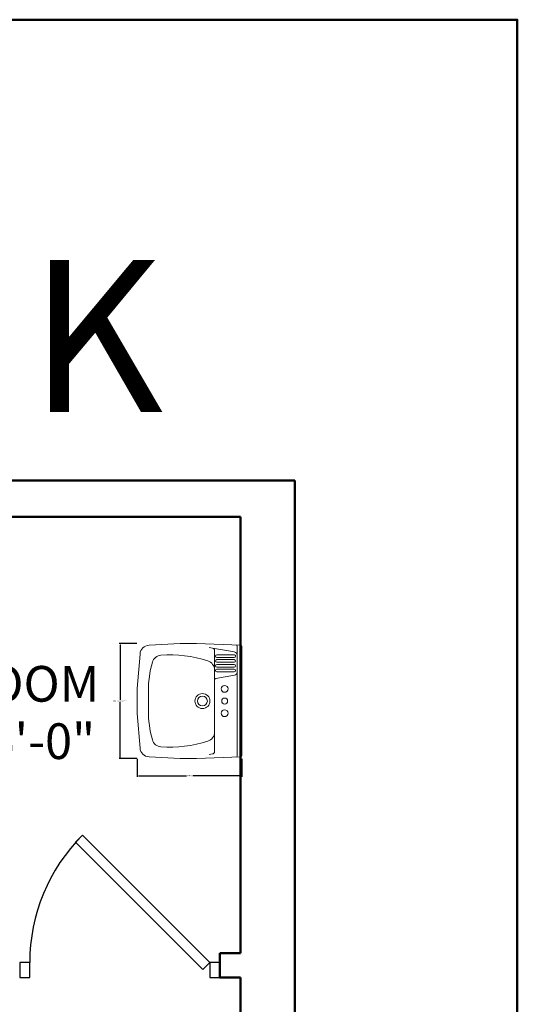
# Model space of a CAD drawing. Units: inches. Extents: x 64 to 1167, y 117 to 939.
# Tile 27 of 56: x 431 to 513, y 777 to 939. Entities that reach past the tile are written whole.
import ezdxf

# ---------------------------------------------------------------- set-up
doc = ezdxf.new("R2010")
doc.units = ezdxf.units.IN
doc.header["$MEASUREMENT"] = 0
for name, color, linetype, lineweight in [('A-ANNO-DIMS', 2, 'Continuous', 18), ('A-ANNO-TEXT', 7, 'Continuous', 25), ('A-ANNO-TTLB', 7, 'Continuous', 50), ('A-DOOR', 4, 'Continuous', 25), ('A-FLOR-FIXT', 8, 'Continuous', 18), ('A-WALL', 7, 'Continuous', 50)]:
    doc.layers.add(name, color=color, linetype=linetype, lineweight=lineweight)
doc.styles.get("Standard").update_dxf_attribs({"font": 'arial.ttf'})
doc.dimstyles.get("Standard").update_dxf_attribs({"dimtxt": 0.18, "dimasz": 0.18, "dimexe": 0.18, "dimexo": 0.0625, "dimgap": 0.09, "dimtad": 0, "dimtih": 1, "dimtoh": 1, "dimdec": 4, "dimzin": 0, "dimdsep": 46, "dimtxsty": 'Standard', "dimcen": 0.09, "dimadec": 0, "dimazin": 0, "dimtfac": 1, "dimtdec": 4, "dimtofl": 0, "dimtmove": 0, "dimatfit": 3, "dimfxl": 1, "dimtolj": 1, "dimtzin": 0, "dimarcsym": 0})

# ---------------------------------------------------------------- blocks, each defined once
blk = doc.blocks.new('A$C68901CC0')
for p, q in [((10.95, 26.62), (12.35, 28.01)), ((12.35, 28.01), (37.4, 2.95)), ((36.01, 1.56), (10.95, 26.62)), ((0, 2.95), (0, 0)), ((1.97, 2.95), (0, 2.95)), ((1.97, 0), (1.97, 2.95)), ((37.4, 2.95), (36.01, 1.56)), ((37.4, 2.95), (37.4, 0)), ((39.37, 2.95), (37.4, 2.95)), ((39.37, 0), (39.37, 2.95)), ((0, 0), (1.97, 0)), ((37.4, 0), (39.37, 0))]:
    blk.add_line(p, q)
blk.add_arc((37.4, 2.95), 35.43, 135, 180)
blk = doc.blocks.new('A$C056A4ABE')
at = {"ltscale": 20}
for p, q in [((0.0065, 0.4339), (0, 0.2479)), ((0.0098, 0.4178), (0.2406, 0.4178)), ((0.2406, 0.4378), (0.0105, 0.4378)), ((0.1205, 0.4178), (0.0475, 0.4178)), ((0.11, 0.4178), (0.0579, 0.4178)), ((0.2406, 0.4378), (0.4708, 0.4378)), ((0.4715, 0.4178), (0.2406, 0.4178)), ((0.4748, 0.4339), (0.4813, 0.2479)), ((0.0188, 0.315), (0.0351, 0.4075)), ((0.0472, 0.4063), (0.0472, 0.3333)), ((0.0582, 0.4063), (0.0582, 0.3333)), ((0.0672, 0.4063), (0.0672, 0.3333)), ((0.0782, 0.4063), (0.0782, 0.3333)), ((0.0872, 0.4063), (0.0872, 0.3333)), ((0.0982, 0.4063), (0.0982, 0.3333)), ((0.1072, 0.4063), (0.1072, 0.3333)), ((0.1182, 0.4063), (0.1182, 0.3333)), ((0.1465, 0.3295), (0.1328, 0.4075)), ((0.0164, 0.3013), (0.0188, 0.315)), ((0.2406, 0.3233), (0.0287, 0.3233)), ((0.2406, 0.3233), (0.1468, 0.3233)), ((0.2406, 0.3233), (0.3344, 0.3233)), ((0.2406, 0.3233), (0.4526, 0.3233)), ((0.4648, 0.3013), (0.4624, 0.315)), ((0, 0.2479), (0, 0.1789)), ((0.4813, 0.2479), (0.4813, 0.1789)), ((0, 0.1789), (0.0068, 0.0492)), ((0.4813, 0.1789), (0.4745, 0.0492)), ((0.2406, 0.0463), (0.2011, 0.0463)), ((0.2406, 0.0463), (0.2802, 0.0463)), ((0.0436, 0.0114), (0.1881, 0)), ((0.1881, 0), (0.2406, 0)), ((0.2932, 0), (0.2406, 0)), ((0.4377, 0.0114), (0.2932, 0))]:
    blk.add_line(p, q, dxfattribs=at)
for centre, radius in [((0.1896, 0.3658), 0.0143), ((0.2406, 0.3658), 0.0125), ((0.2916, 0.3658), 0.0143), ((0.2406, 0.2728), 0.0315), ((0.2406, 0.2728), 0.0205)]:
    blk.add_circle(centre, radius, dxfattribs=at)
for centre, radius, start, end in [((0.0098, 0.4138), 0.004, 90, 178), ((0.0105, 0.4338), 0.004, 90, 178), ((0.0475, 0.4053), 0.0125, 90, 170), ((0.1205, 0.4053), 0.0125, 10, 90), ((0.4708, 0.4338), 0.004, 2, 90), ((0.4715, 0.4138), 0.004, 2, 90), ((0.0527, 0.4063), 0.0055, 0, 172.1464), ((0.0727, 0.4063), 0.0055, 0, 180), ((0.0927, 0.4063), 0.0055, 0, 180), ((0.1127, 0.4063), 0.0055, 0, 180), ((0.0527, 0.3333), 0.0055, 180, 0), ((0.0727, 0.3333), 0.0055, 180, 0), ((0.0927, 0.3333), 0.0055, 180, 0), ((0.1127, 0.3333), 0.0055, 180, 0), ((0.0287, 0.3133), 0.01, 90, 170), ((0.5633, 0.1363), 0.516, 162.0492, 184.1817), ((0.1106, 0.2833), 0.04, 90, 162.5107), ((0.1539, 0.3308), 0.0075, 190, 270), ((0.3706, 0.2833), 0.04, 17.4893, 90), ((-0.0821, 0.1363), 0.516, 355.8183, 17.9508), ((0.4526, 0.3133), 0.01, 10, 90), ((0.0886, 0.1016), 0.04, 184.1813, 254.5087), ((0.3926, 0.1016), 0.04, 285.4913, 355.8187), ((0.0467, 0.0512), 0.04, 183, 265.5), ((0.2011, 0.5073), 0.461, 254.5087, 270), ((0.2802, 0.5073), 0.461, 270, 285.4913), ((0.4345, 0.0512), 0.04, 274.5, 357)]:
    blk.add_arc(centre, radius, start, end, dxfattribs=at)
blk = doc.blocks.new('*D68')
at = {"layer": 'A-ANNO-DIMS', "color": 0, "lineweight": -2, "transparency": 16777216}
for p, q in [((450.05, 836.28), (447.09, 836.28)), ((447.27, 836.1), (447.27, 826.99)), ((447.27, 817.51), (447.27, 826.62)), ((450.05, 817.33), (447.09, 817.33))]:
    blk.add_line(p, q, dxfattribs=at)
for points in [[(447.24, 836.1), (447.3, 836.1), (447.27, 836.28)], [(447.24, 817.51), (447.3, 817.51), (447.27, 817.33)]]:
    blk.add_solid(points, dxfattribs=at)
at = {"layer": 'Defpoints', "color": 0, "lineweight": -2, "transparency": 16777216}
for p in [(450.11, 836.28), (447.27, 817.33), (450.11, 817.33)]:
    blk.add_point(p, dxfattribs=at)
at = {"layer": 'A-ANNO-DIMS', "color": 0, "transparency": 16777216, "insert": (447.27, 826.81), "char_height": 0.18, "attachment_point": 5}
blk.add_mtext('\\A1;WASH BASIN 19 TYP.', dxfattribs=at)
blk = doc.blocks.new('*D69')
at = {"layer": 'A-ANNO-DIMS', "color": 0, "lineweight": -2, "transparency": 16777216}
for p, q in [((450.11, 817.27), (450.11, 814.31)), ((467.35, 817.27), (467.35, 814.31)), ((450.29, 814.49), (458.21, 814.49)), ((467.17, 814.49), (459.25, 814.49))]:
    blk.add_line(p, q, dxfattribs=at)
for points in [[(450.29, 814.52), (450.29, 814.46), (450.11, 814.49)], [(467.17, 814.52), (467.17, 814.46), (467.35, 814.49)]]:
    blk.add_solid(points, dxfattribs=at)
at = {"layer": 'Defpoints', "color": 0, "lineweight": -2, "transparency": 16777216}
for p in [(450.11, 817.33), (467.35, 817.33), (467.35, 814.49)]:
    blk.add_point(p, dxfattribs=at)
at = {"layer": 'A-ANNO-DIMS', "color": 0, "transparency": 16777216, "insert": (458.73, 814.49), "char_height": 0.18, "attachment_point": 5}
blk.add_mtext('\\A1;17 TYP.', dxfattribs=at)

msp = doc.modelspace()

# ---------------------------------------------------------------- linework, layer by layer
at = {"layer": 'A-ANNO-TTLB'}
msp.add_lwpolyline([(64.31, 939.22), (512.77, 939.22), (512.77, 116.55), (64.31, 116.55)], close=True, dxfattribs=at)
at = {"layer": 'A-WALL'}
for p, q in [((476.11, 863.2), (122.11, 863.2)), ((476.11, 863.2), (476.11, 155.2)), ((467.11, 857.2), (377.11, 857.2)), ((467.11, 857.2), (467.11, 785.2)), ((467.11, 785.2), (463.72, 785.2)), ((463.72, 781.2), (463.72, 785.2)), ((467.11, 781.2), (463.72, 781.2)), ((467.11, 781.2), (467.11, 637.2))]:
    msp.add_line(p, q, dxfattribs=at)

# ---------------------------------------------------------------- block references
at = {"layer": 'A-DOOR', "xscale": 0.8381879042225197, "yscale": 0.8381879042225197, "zscale": 0.8381879042225197}
msp.add_blockref('A$C68901CC0', (430.72, 781.2), dxfattribs=at)
at = {"layer": 'A-FLOR-FIXT', "xscale": 39.37007874015748, "yscale": 39.37007874015748, "zscale": 39.37007874015748, "rotation": 270.0000000032171}
msp.add_blockref('A$C056A4ABE', (450.11, 836.28), dxfattribs=at)

# ---------------------------------------------------------------- texts
at = {"layer": 'A-ANNO-TEXT'}
for s, height, p in [('FLOOR PLAN OF 3BHK', 25.0713, (102.99, 874.51)), ('BATH ROOM', 5.893, (397.64, 826.7)), (' 7\'-6" X 6\'-0"', 5.8926, (397.64, 817.24))]:
    msp.add_text(s, height=height, dxfattribs=at).set_placement(p)

# ---------------------------------------------------------------- dimensions: what is measured, and where the dimension line sits
at = {"layer": 'A-ANNO-DIMS'}
for base, p1, p2, angle, text, picture, middle in [((447.27, 817.33), (450.11, 836.28), (450.11, 817.33), 270, 'WASH BASIN <> TYP.', '*D68', (447.27, 826.81)), ((467.35, 814.49), (450.11, 817.33), (467.35, 817.33), 0, '<> TYP.', '*D69', (458.73, 814.49))]:
    dim = msp.add_linear_dim(base=base, p1=p1, p2=p2, angle=angle, text=text, dimstyle='Standard', override={"dimdec": 0, "dimlfac": 1, "dimrnd": 0, "dimzin": 0, "dimdsep": 46, "dimlunit": 2}, dxfattribs=at)
    dim.commit()
    dim.dimension.update_dxf_attribs({"geometry": picture, "text_midpoint": middle})

doc.saveas('drawing.dxf')
